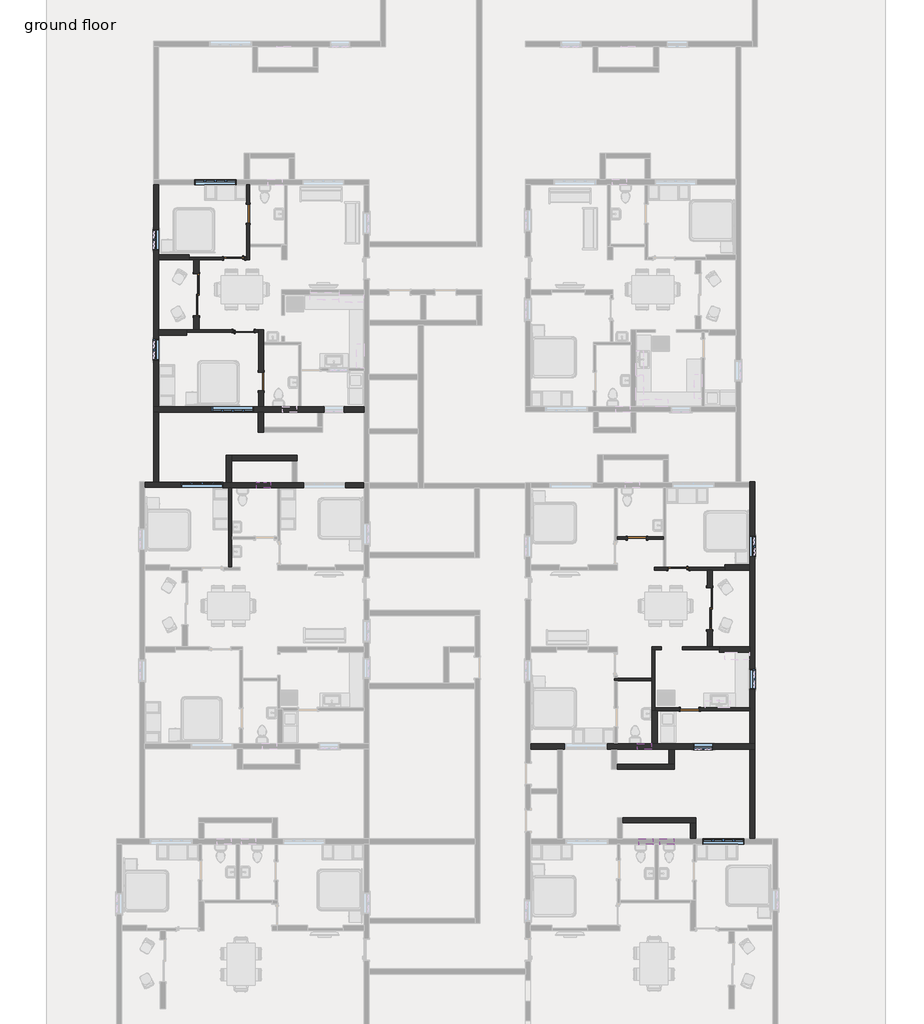
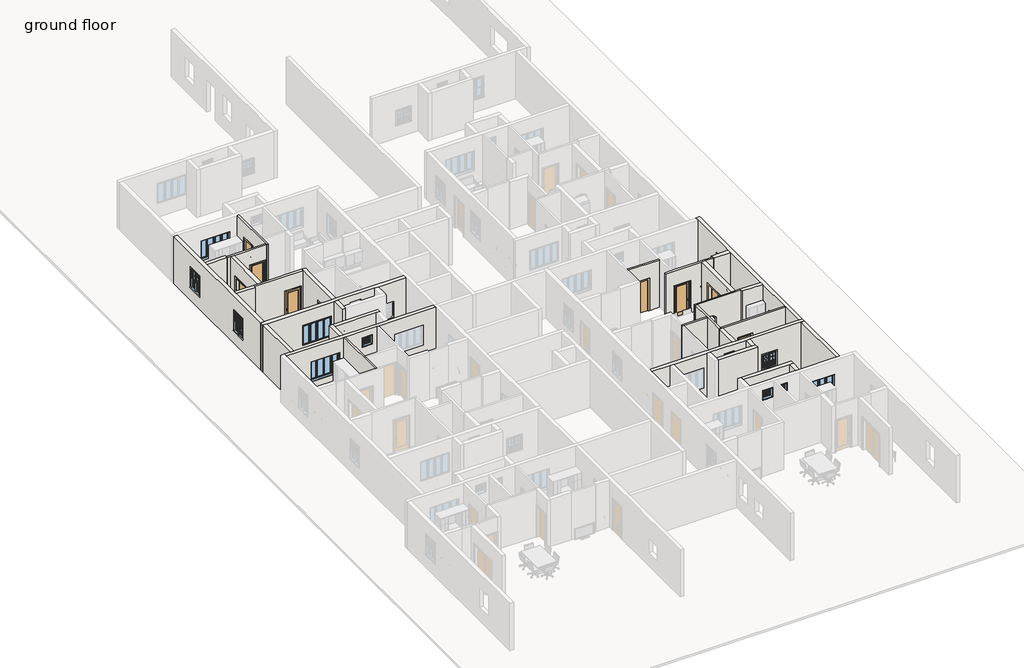
# One storey, part 4 of 16: 32 walls, 13 windows, 9 doors.
"""IFC4 building model written with IfcOpenShell, lengths in millimetres."""

from ifc_helpers import new_model, si_unit, point, frame, origin, place, context, project, spatial, polyline, ellipse_curve, trimmed, outline, extrude, faceted_brep, transform, mapped, element, save
from ifc_brep_helpers import plane_surface, extruded_surface, advanced_brep
from components import door_d4d75d1e, door_a3feeac7, door_38851409, door_d141acb4, door_7b345704, window_ced37e8f, window_5487fb6d, window_f2d8fef0, window_45970670

model = new_model("IFC4")

# Units and contexts
model_context = context("Model", 3, world=origin())
ifc_project = project(units=[si_unit("LENGTHUNIT", "METRE", prefix="MILLI")], contexts=[model_context])

# Site, building, storey
site = spatial("IfcSite", under=ifc_project)
building = spatial("IfcBuilding", under=site)
storey = spatial("IfcBuildingStorey", under=building, Name="ground floor", Elevation=609.6)

# Doors
placement = place(None, origin())
door_shape = door_d4d75d1e(model_context)
element("IfcDoor", 1, ObjectType="Door-Double-Sliding : 72\" x 84\"", at=placement, inside=storey, context=model_context, shape_type="MappedRepresentation", body=[
    mapped(door_shape, transform((67268.6312819, -3471.0113664, 609.6), x_axis=(0.0, -1.0, 0.0), y_axis=(1.0, 0.0, 0.0), z_axis=(0.0, 0.0, 1.0))),
])
element("IfcDoor", 2, ObjectType="Door-Double-Sliding : 72\" x 84\"", at=placement, inside=storey, context=model_context, shape_type="MappedRepresentation", body=[
    mapped(door_shape, transform((44881.526243, 10200.7650652, 609.6), x_axis=(0.0, -1.0, 0.0), y_axis=(1.0, 0.0, 0.0), z_axis=(0.0, 0.0, 1.0))),
])
door_2_shape = door_a3feeac7(model_context)
element("IfcDoor", 3, ObjectType="Door-Interior-Single-1_Panel-Wood : 36\" x 84\"", at=placement, inside=storey, context=model_context, shape_type="MappedRepresentation", body=[
    mapped(door_2_shape, transform((46653.176243, 11785.0900652, 609.6), x_axis=(-1.0, 0.0, 0.0), y_axis=(0.0, -1.0, 0.0), z_axis=(0.0, 0.0, 1.0))),
])
element("IfcDoor", 4, ObjectType="Door-Interior-Single-1_Panel-Wood : 36\" x 84\"", at=placement, inside=storey, context=model_context, shape_type="MappedRepresentation", body=[
    mapped(door_2_shape, transform((47065.926243, 8616.4400652, 609.6), x_axis=(1.0, 0.0, 0.0), y_axis=(0.0, 1.0, 0.0), z_axis=(0.0, 0.0, 1.0))),
])
element("IfcDoor", 5, ObjectType="Door-Interior-Single-1_Panel-Wood : 36\" x 84\"", at=placement, inside=storey, context=model_context, shape_type="MappedRepresentation", body=[
    mapped(door_2_shape, transform((66030.3812819, -1734.2863664, 609.6), x_axis=(-1.0, 0.0, 0.0), y_axis=(0.0, -1.0, 0.0), z_axis=(0.0, 0.0, 1.0))),
])
door_3_shape = door_38851409(model_context)
element("IfcDoor", 6, ObjectType="Single-Flush : 32\" x 84\"", at=placement, inside=storey, context=model_context, shape_type="MappedRepresentation", body=[
    mapped(door_3_shape, transform((64214.2812819, -403.9613664, 609.6), x_axis=(-1.0, 0.0, 0.0), y_axis=(0.0, -1.0, 0.0), z_axis=(0.0, 0.0, 1.0))),
])
door_4_shape = door_d141acb4(model_context)
element("IfcDoor", 7, ObjectType="Single-Flush : 32\" x 84\"", at=placement, inside=storey, context=model_context, shape_type="MappedRepresentation", body=[
    mapped(door_4_shape, transform((47262.776243, 13732.8934407, 609.6), x_axis=(0.0, -1.0, 0.0), y_axis=(1.0, 0.0, 0.0), z_axis=(0.0, 0.0, 1.0))),
])
element("IfcDoor", 8, ObjectType="Single-Flush : 32\" x 84\"", at=placement, inside=storey, context=model_context, shape_type="MappedRepresentation", body=[
    mapped(door_4_shape, transform((66519.3312819, -7858.8613664, 609.6), x_axis=(-1.0, 0.0, 0.0), y_axis=(0.0, -1.0, 0.0), z_axis=(0.0, 0.0, 1.0))),
])
door_5_shape = door_7b345704(model_context)
element("IfcDoor", 9, ObjectType="Single-Flush : 32\" x 84\"", at=placement, inside=storey, context=model_context, shape_type="MappedRepresentation", body=[
    mapped(door_5_shape, transform((47827.926243, 6425.5718163, 609.6), x_axis=(0.0, 1.0, 0.0), y_axis=(-1.0, 0.0, 0.0), z_axis=(0.0, 0.0, 1.0))),
])

# Walls
element("IfcWall", 10, ObjectType="Generic - 4.5\"", at=placement, inside=storey, context=model_context, shape_type="Brep", body=[
    faceted_brep([(47205.626243, 13326.4934407, 2743.2), (47205.626243, 13326.4934407, 609.6), (47205.626243, 11839.0650652, 609.6), (47205.626243, 11724.7650652, 609.6), (47205.626243, 11724.7650652, 3810.0), (47205.626243, 11839.0650652, 3810.0), (47205.626243, 14998.0718163, 3810.0), (47205.626243, 14998.0718163, 609.6), (47205.626243, 14139.2934407, 609.6), (47205.626243, 14139.2934407, 2743.2), (47319.926243, 11724.7650652, 609.6), (47319.926243, 12296.2650652, 609.6), (47319.926243, 12410.5650652, 609.6), (47319.926243, 13326.4934407, 609.6), (47319.926243, 13326.4934407, 2743.2), (47319.926243, 14139.2934407, 2743.2), (47319.926243, 14139.2934407, 609.6), (47319.926243, 14998.0718163, 609.6), (47319.926243, 14998.0718163, 3810.0), (47319.926243, 12410.5650652, 3810.0), (47319.926243, 12296.2650652, 3810.0), (47319.926243, 11724.7650652, 3810.0)], [[[0, 1, 2, 3, 4, 5, 6, 7, 8, 9]], [[10, 11, 12, 13, 14, 15, 16, 17, 18, 19, 20, 21]], [[8, 7, 17, 16]], [[3, 2, 1, 13, 12, 11, 10]], [[6, 5, 4, 21, 20, 19, 18]], [[7, 6, 18, 17]], [[4, 3, 10, 21]], [[14, 13, 1, 0]], [[15, 14, 0, 9]], [[16, 15, 9, 8]]]),
])
element("IfcWall", 11, ObjectType="Generic - 4.5\"", at=placement, inside=storey, context=model_context, shape_type="Brep", body=[
    faceted_brep([(47205.626243, 11724.7650652, 3810.0), (45122.826243, 11724.7650652, 3810.0), (44894.226243, 11724.7650652, 3810.0), (44680.0946956, 11724.7650652, 3810.0), (44680.0946956, 11724.7650652, 609.6), (44894.226243, 11724.7650652, 609.6), (45122.826243, 11724.7650652, 609.6), (46170.576243, 11724.7650652, 609.6), (46170.576243, 11724.7650652, 2768.6), (47135.776243, 11724.7650652, 2768.6), (47135.776243, 11724.7650652, 609.6), (47205.626243, 11724.7650652, 609.6), (44680.0946956, 11839.0650652, 3810.0), (47205.626243, 11839.0650652, 3810.0), (47205.626243, 11839.0650652, 609.6), (47135.776243, 11839.0650652, 609.6), (47135.776243, 11839.0650652, 2768.6), (46170.576243, 11839.0650652, 2768.6), (46170.576243, 11839.0650652, 609.6), (44680.0946956, 11839.0650652, 609.6)], [[[0, 1, 2, 3, 4, 5, 6, 7, 8, 9, 10, 11]], [[12, 13, 14, 15, 16, 17, 18, 19]], [[4, 19, 18, 7, 6, 5]], [[14, 11, 10, 15]], [[3, 2, 1, 0, 13, 12]], [[4, 3, 12, 19]], [[0, 11, 14, 13]], [[17, 8, 7, 18]], [[8, 17, 16, 9]], [[9, 16, 15, 10]]]),
])
element("IfcWall", 12, ObjectType="Generic - 4.5\"", at=placement, inside=storey, context=model_context, shape_type="Brep", body=[
    faceted_brep([(47713.626243, 8562.4650652, 3810.0), (44589.426243, 8562.4650652, 3810.0), (44589.426243, 8562.4650652, 609.6), (46583.326243, 8562.4650652, 609.6), (46583.326243, 8562.4650652, 2768.6), (47548.526243, 8562.4650652, 2768.6), (47548.526243, 8562.4650652, 609.6), (47713.626243, 8562.4650652, 609.6), (44589.426243, 8676.7650652, 3810.0), (44894.226243, 8676.7650652, 3810.0), (45122.826243, 8676.7650652, 3810.0), (47713.626243, 8676.7650652, 3810.0), (47713.626243, 8676.7650652, 609.6), (47548.526243, 8676.7650652, 609.6), (47548.526243, 8676.7650652, 2768.6), (46583.326243, 8676.7650652, 2768.6), (46583.326243, 8676.7650652, 609.6), (45122.826243, 8676.7650652, 609.6), (44894.226243, 8676.7650652, 609.6), (44589.426243, 8676.7650652, 609.6)], [[[0, 1, 2, 3, 4, 5, 6, 7]], [[8, 9, 10, 11, 12, 13, 14, 15, 16, 17, 18, 19]], [[2, 19, 18, 17, 16, 3]], [[12, 7, 6, 13]], [[1, 0, 11, 10, 9, 8]], [[2, 1, 8, 19]], [[0, 7, 12, 11]], [[5, 14, 13, 6]], [[14, 5, 4, 15]], [[15, 4, 3, 16]]]),
])
element("IfcWall", 13, ObjectType="Generic - 4.5\"", at=placement, inside=storey, context=model_context, shape_type="Brep", body=[
    faceted_brep([(46418.226243, 1802.8108651, 609.6), (46418.226243, -1680.3113664, 609.6), (46418.226243, -1680.3113664, 3810.0), (46418.226243, 1802.8108651, 3810.0), (46532.526243, 1802.356101, 609.6), (46532.526243, 1802.356101, 3810.0), (46532.526243, -346.8113664, 3810.0), (46532.526243, -461.1113664, 3810.0), (46532.526243, -1680.3113664, 3810.0), (46532.526243, -1680.3113664, 609.6), (46532.526243, -461.1113664, 609.6), (46532.526243, -346.8113664, 609.6)], [[[0, 1, 2, 3]], [[4, 5, 6, 7, 8, 9, 10, 11]], [[1, 0, 4, 11, 10, 9]], [[3, 2, 8, 7, 6, 5]], [[0, 3, 5, 4]], [[2, 1, 9, 8]]]),
])
element("IfcWall", 14, ObjectType="Generic - 4.5\"", at=placement, inside=storey, context=model_context, shape_type="SweptSolid", body=[
    extrude(outline(polyline([(609.6, 63357.0312819), (609.6, 63807.8812819), (2743.2, 63807.8812819), (2743.2, 64620.6812819), (609.6, 64620.6812819), (609.6, 65363.6312819), (3810.0, 65363.6312819), (3810.0, 63357.0312819), (609.6, 63357.0312819)])), frame((0.0, -461.1113664, 0.0), z_axis=(0.0, 1.0, 0.0), x_axis=(0.0, 0.0, 1.0)), (0.0, 0.0, 1.0), 114.3),
])
element("IfcWall", 15, ObjectType="Generic - 4.5\"", at=placement, inside=storey, context=model_context, shape_type="Brep", body=[
    faceted_brep([(64971.2300724, -1680.3113664, 609.6), (64971.2300724, -1680.3113664, 3810.0), (65363.6312819, -1680.3113664, 3810.0), (65477.9312819, -1680.3113664, 3810.0), (68044.6300724, -1680.3113664, 3810.0), (68044.6300724, -1680.3113664, 609.6), (66512.9812819, -1680.3113664, 609.6), (66512.9812819, -1680.3113664, 2768.6), (65547.7812819, -1680.3113664, 2768.6), (65547.7812819, -1680.3113664, 609.6), (65477.9312819, -1680.3113664, 609.6), (65363.6312819, -1680.3113664, 609.6), (64971.2300724, -1794.6113664, 3810.0), (64971.2300724, -1794.6113664, 609.6), (65547.7812819, -1794.6113664, 609.6), (65547.7812819, -1794.6113664, 2768.6), (66512.9812819, -1794.6113664, 2768.6), (66512.9812819, -1794.6113664, 609.6), (67281.3312819, -1794.6113664, 609.6), (67509.9312819, -1794.6113664, 609.6), (68044.6300724, -1794.6113664, 609.6), (68044.6300724, -1794.6113664, 3810.0), (67509.9312819, -1794.6113664, 3810.0), (67281.3312819, -1794.6113664, 3810.0)], [[[0, 1, 2, 3, 4, 5, 6, 7, 8, 9, 10, 11]], [[12, 13, 14, 15, 16, 17, 18, 19, 20, 21, 22, 23]], [[13, 0, 11, 10, 9, 14]], [[5, 20, 19, 18, 17, 6]], [[1, 0, 13, 12]], [[4, 3, 2, 1, 12, 23, 22, 21]], [[5, 4, 21, 20]], [[8, 15, 14, 9]], [[15, 8, 7, 16]], [[16, 7, 6, 17]]]),
])
element("IfcWall", 16, ObjectType="Generic - 4.5\"", at=placement, inside=storey, context=model_context, shape_type="AdvancedBrep", body=[
    advanced_brep(
    [(65293.7812819, -5147.4113664, 2540.0), (65293.7812819, -5147.4113664, 609.6), (64881.0312819, -5147.4113664, 609.6), (64881.0312819, -5147.4113664, 3810.0), (67281.3312819, -5147.4113664, 3810.0), (67509.9312819, -5147.4113664, 3810.0), (67802.0312819, -5147.4113664, 3810.0), (67802.0312819, -5147.4113664, 609.6), (67509.9312819, -5147.4113664, 609.6), (67281.3312819, -5147.4113664, 609.6), (66208.1812819, -5147.4113664, 609.6), (66208.1812819, -5147.4113664, 2540.0), (64881.0312819, -5261.7113664, 609.6), (64995.3312819, -5261.7113664, 609.6), (65293.7812819, -5261.7113664, 609.6), (65293.7812819, -5261.7113664, 2540.0), (66208.1812819, -5261.7113664, 2540.0), (66208.1812819, -5261.7113664, 609.6), (67802.0312819, -5261.7113664, 609.6), (67802.0312819, -5261.7113664, 3810.0), (64995.3312819, -5261.7113664, 3810.0), (64881.0312819, -5261.7113664, 3810.0)],
    [
        (0, 1),
        (1, 2),
        (2, 3),
        (3, 4),
        (4, 5),
        (5, 6),
        (6, 7),
        (7, 8),
        (8, 9),
        (9, 10),
        (10, 11),
        (11, 0, ellipse_curve(frame((65750.9812819, -5147.4113664, 2540.0), z_axis=(0.0, -1.0, 0.0), x_axis=(-1.0, 0.0, 0.0)), 457.2, 203.2)),
        (12, 13),
        (13, 14),
        (14, 15),
        (15, 16, ellipse_curve(frame((65750.9812819, -5261.7113664, 2540.0), z_axis=(0.0, 1.0, 0.0), x_axis=(-1.0, 0.0, 0.0)), 457.2, 203.2)),
        (16, 17),
        (17, 18),
        (18, 19),
        (19, 20),
        (20, 21),
        (21, 12),
        (1, 14),
        (12, 2),
        (7, 18),
        (17, 10),
        (3, 21),
        (19, 6),
        (15, 0),
        (11, 16),
    ],
    [
        plane_surface(frame((67798.9718682, -5147.4113664, 609.6), z_axis=(0.0, 1.0, 0.0), x_axis=(-1.0, 0.0, 0.0))),
        plane_surface(frame((67798.9718682, -5261.7113664, 609.6), z_axis=(0.0, -1.0, 0.0), x_axis=(1.0, 0.0, 0.0))),
        plane_surface(frame((67802.0312819, -5147.4113664, 609.6), z_axis=(0.0, 0.0, -1.0), x_axis=(0.0, -1.0, 0.0))),
        plane_surface(frame((64938.1812819, -5147.4113664, 3810.0), z_axis=(0.0, 0.0, 1.0), x_axis=(0.0, -1.0, 0.0))),
        plane_surface(frame((67802.0312819, -5147.4113664, 3810.0), z_axis=(1.0, 0.0, 0.0), x_axis=(0.0, -1.0, 0.0))),
        plane_surface(frame((64881.0312819, -5147.4113664, 609.6), z_axis=(-1.0, 0.0, 0.0), x_axis=(0.0, -1.0, 0.0))),
        extruded_surface(trimmed(ellipse_curve(frame((65750.9812819, -5033.1113664, 2540.0), z_axis=(0.0, 1.0, 0.0), x_axis=(-1.0, 0.0, 0.0)), 457.2, 203.2), [point((65293.7812819, -5033.1113664, 2540.0))], [point((66208.1812819, -5033.1113664, 2540.0))], True, "CARTESIAN"), (0.0, -114.29999999999927, 0.0), 114.29999999999927),
        plane_surface(frame((66208.1812819, -5261.7113664, 2540.0), z_axis=(-1.0, 0.0, 0.0), x_axis=(0.0, 1.0, 0.0))),
        plane_surface(frame((65293.7812819, -5261.7113664, 609.6), z_axis=(1.0, 0.0, 0.0), x_axis=(0.0, 1.0, 0.0))),
    ],
    [
        (0, [[1, 2, 3, 4, 5, 6, 7, 8, 9, 10, 11, 12]]),
        (1, [[13, 14, 15, 16, 17, 18, 19, 20, 21, 22]]),
        (2, [[-2, 23, -14, -13, 24]]),
        (2, [[-10, -9, -8, 25, -18, 26]]),
        (3, [[-6, -5, -4, 27, -21, -20, 28]]),
        (4, [[-7, -28, -19, -25]]),
        (5, [[-3, -24, -22, -27]]),
        (6, [[-16, 29, -12, 30]]),
        (7, [[-17, -30, -11, -26]]),
        (8, [[-15, -23, -1, -29]]),
    ],
),
])
element("IfcWall", 17, ObjectType="Generic - 4.5\"", at=placement, inside=storey, context=model_context, shape_type="Brep", body=[
    faceted_brep([(64881.0312819, -5261.7113664, 609.6), (64881.0312819, -6506.3113664, 609.6), (64881.0312819, -6620.6113664, 609.6), (64881.0312819, -7916.0113664, 609.6), (64881.0312819, -7916.0113664, 3810.0), (64881.0312819, -6620.6113664, 3810.0), (64881.0312819, -6506.3113664, 3810.0), (64881.0312819, -5261.7113664, 3810.0), (64995.3312819, -5261.7113664, 609.6), (64995.3312819, -5261.7113664, 3810.0), (64995.3312819, -7801.7113664, 3810.0), (64995.3312819, -7916.0113664, 3810.0), (64995.3312819, -7916.0113664, 609.6), (64995.3312819, -7801.7113664, 609.6)], [[[0, 1, 2, 3, 4, 5, 6, 7]], [[8, 9, 10, 11, 12, 13]], [[3, 2, 1, 0, 8, 13, 12]], [[7, 6, 5, 4, 11, 10, 9]], [[0, 7, 9, 8]], [[4, 3, 12, 11]]]),
])
element("IfcWall", 18, ObjectType="Generic - 4.5\"", at=placement, inside=storey, context=model_context, shape_type="Brep", body=[
    faceted_brep([(64995.3312819, -7916.0113664, 609.6), (65109.6312819, -7916.0113664, 609.6), (66112.9312819, -7916.0113664, 609.6), (66112.9312819, -7916.0113664, 2743.2), (66925.7312819, -7916.0113664, 2743.2), (66925.7312819, -7916.0113664, 609.6), (69135.5312819, -7916.0113664, 609.6), (69135.5312819, -7916.0113664, 3810.0), (65109.6312819, -7916.0113664, 3810.0), (64995.3312819, -7916.0113664, 3810.0), (66112.9312819, -7801.7113664, 2743.2), (66112.9312819, -7801.7113664, 609.6), (64995.3312819, -7801.7113664, 609.6), (64995.3312819, -7801.7113664, 3810.0), (69135.5312819, -7801.7113664, 3810.0), (69135.5312819, -7801.7113664, 609.6), (66925.7312819, -7801.7113664, 609.6), (66925.7312819, -7801.7113664, 2743.2)], [[[0, 1, 2, 3, 4, 5, 6, 7, 8, 9]], [[10, 11, 12, 13, 14, 15, 16, 17]], [[16, 15, 6, 5]], [[12, 11, 2, 1, 0]], [[9, 8, 7, 14, 13]], [[0, 9, 13, 12]], [[7, 6, 15, 14]], [[3, 2, 11, 10]], [[4, 3, 10, 17]], [[5, 4, 17, 16]]]),
])
element("IfcWall", 19, ObjectType="Generic - 4.5\"", at=placement, inside=storey, context=model_context, shape_type="Brep", body=[
    faceted_brep([(64881.0312819, -6506.3113664, 609.6), (63357.0312819, -6506.3113664, 609.6), (63242.7312819, -6506.3113664, 609.6), (63242.7312819, -6506.3113664, 3810.0), (63357.0312819, -6506.3113664, 3810.0), (64881.0312819, -6506.3113664, 3810.0), (64881.0312819, -6620.6113664, 609.6), (64881.0312819, -6620.6113664, 3810.0), (63357.0312819, -6620.6113664, 3810.0), (63242.7312819, -6620.6113664, 3810.0), (63242.7312819, -6620.6113664, 609.6), (63357.0312819, -6620.6113664, 609.6)], [[[0, 1, 2, 3, 4, 5]], [[6, 7, 8, 9, 10, 11]], [[2, 1, 0, 6, 11, 10]], [[5, 4, 3, 9, 8, 7]], [[0, 5, 7, 6]], [[3, 2, 10, 9]]]),
])
element("IfcWall", 20, ObjectType="Generic - 9\"", at=placement, inside=storey, context=model_context, shape_type="Brep", body=[
    faceted_brep([(52311.026243, 5320.6718163, 609.6), (49580.526243, 5320.6718163, 609.6), (49466.226243, 5320.6718163, 609.6), (47942.226243, 5320.6718163, 609.6), (47713.626243, 5320.6718163, 609.6), (43370.226243, 5320.6718163, 609.6), (43141.626243, 5320.6718163, 609.6), (43141.626243, 5320.6718163, 3810.0), (43370.226243, 5320.6718163, 3810.0), (47713.626243, 5320.6718163, 3810.0), (47942.226243, 5320.6718163, 3810.0), (49466.226243, 5320.6718163, 3810.0), (49580.526243, 5320.6718163, 3810.0), (52311.026243, 5320.6718163, 3810.0), (45681.626243, 5320.6718163, 2870.2), (45681.626243, 5320.6718163, 1524.0), (47510.426243, 5320.6718163, 1524.0), (47510.426243, 5320.6718163, 2870.2), (50583.295833, 5320.6718163, 2438.4), (50583.295833, 5320.6718163, 1524.0), (51446.895833, 5320.6718163, 1524.0), (51446.895833, 5320.6718163, 2438.4), (49370.976243, 5320.6718163, 3352.8), (48761.376243, 5320.6718163, 3352.8), (48761.376243, 5320.6718163, 2743.2), (49370.976243, 5320.6718163, 2743.2), (52311.026243, 5092.0718163, 609.6), (52311.026243, 5092.0718163, 3810.0), (50519.795833, 5092.0718163, 3810.0), (50291.195833, 5092.0718163, 3810.0), (47929.526243, 5092.0718163, 3810.0), (47700.926243, 5092.0718163, 3810.0), (43370.226243, 5092.0718163, 3810.0), (43141.626243, 5092.0718163, 3810.0), (43141.626243, 5092.0718163, 609.6), (43370.226243, 5092.0718163, 609.6), (47700.926243, 5092.0718163, 609.6), (47929.526243, 5092.0718163, 609.6), (50291.195833, 5092.0718163, 609.6), (50519.795833, 5092.0718163, 609.6), (45681.626243, 5092.0718163, 2870.2), (47510.426243, 5092.0718163, 2870.2), (47510.426243, 5092.0718163, 1524.0), (45681.626243, 5092.0718163, 1524.0), (50583.295833, 5092.0718163, 2438.4), (51446.895833, 5092.0718163, 2438.4), (51446.895833, 5092.0718163, 1524.0), (50583.295833, 5092.0718163, 1524.0), (49370.976243, 5092.0718163, 3352.8), (49370.976243, 5092.0718163, 2743.2), (48761.376243, 5092.0718163, 2743.2), (48761.376243, 5092.0718163, 3352.8)], [[[0, 1, 2, 3, 4, 5, 6, 7, 8, 9, 10, 11, 12, 13], [14, 15, 16, 17], [18, 19, 20, 21], [22, 23, 24, 25]], [[26, 27, 28, 29, 30, 31, 32, 33, 34, 35, 36, 37, 38, 39], [40, 41, 42, 43], [44, 45, 46, 47], [48, 49, 50, 51]], [[6, 5, 4, 3, 2, 1, 0, 26, 39, 38, 37, 36, 35, 34]], [[13, 12, 11, 10, 9, 8, 7, 33, 32, 31, 30, 29, 28, 27]], [[0, 13, 27, 26]], [[7, 6, 34, 33]], [[15, 14, 40, 43]], [[16, 15, 43, 42]], [[17, 16, 42, 41]], [[14, 17, 41, 40]], [[19, 18, 44, 47]], [[20, 19, 47, 46]], [[21, 20, 46, 45]], [[18, 21, 45, 44]], [[49, 48, 22, 25]], [[50, 49, 25, 24]], [[51, 50, 24, 23]], [[48, 51, 23, 22]]]),
])
element("IfcWall", 21, ObjectType="Generic - 9\"", at=placement, inside=storey, context=model_context, shape_type="Brep", body=[
    faceted_brep([(43370.226243, 5320.6718163, 609.6), (43370.226243, 8448.1650652, 609.6), (43370.226243, 8676.7650652, 609.6), (43370.226243, 11724.7650652, 609.6), (43370.226243, 11953.3650652, 609.6), (43370.226243, 14998.0718163, 609.6), (43370.226243, 14998.0718163, 3810.0), (43370.226243, 11953.3650652, 3810.0), (43370.226243, 11724.7650652, 3810.0), (43370.226243, 8676.7650652, 3810.0), (43370.226243, 8448.1650652, 3810.0), (43370.226243, 5320.6718163, 3810.0), (43370.226243, 7343.2650652, 2844.8), (43370.226243, 8257.6650652, 2844.8), (43370.226243, 8257.6650652, 1524.0), (43370.226243, 7343.2650652, 1524.0), (43370.226243, 12143.8650652, 2844.8), (43370.226243, 13058.2650652, 2844.8), (43370.226243, 13058.2650652, 1524.0), (43370.226243, 12143.8650652, 1524.0), (43141.626243, 5320.6718163, 609.6), (43141.626243, 5320.6718163, 3810.0), (43141.626243, 14998.0718163, 3810.0), (43141.626243, 14998.0718163, 609.6), (43141.626243, 7343.2650652, 2844.8), (43141.626243, 7343.2650652, 1524.0), (43141.626243, 8257.6650652, 1524.0), (43141.626243, 8257.6650652, 2844.8), (43141.626243, 12143.8650652, 2844.8), (43141.626243, 12143.8650652, 1524.0), (43141.626243, 13058.2650652, 1524.0), (43141.626243, 13058.2650652, 2844.8)], [[[0, 1, 2, 3, 4, 5, 6, 7, 8, 9, 10, 11], [12, 13, 14, 15], [16, 17, 18, 19]], [[20, 21, 22, 23], [24, 25, 26, 27], [28, 29, 30, 31]], [[5, 4, 3, 2, 1, 0, 20, 23]], [[11, 10, 9, 8, 7, 6, 22, 21]], [[6, 5, 23, 22]], [[0, 11, 21, 20]], [[25, 24, 12, 15]], [[26, 25, 15, 14]], [[27, 26, 14, 13]], [[24, 27, 13, 12]], [[29, 28, 16, 19]], [[30, 29, 19, 18]], [[31, 30, 18, 17]], [[28, 31, 17, 16]]]),
])
element("IfcWall", 22, ObjectType="Generic - 9\"", at=placement, inside=storey, context=model_context, shape_type="Brep", body=[
    faceted_brep([(43370.226243, 11724.7650652, 609.6), (44680.0946956, 11724.7650652, 609.6), (44680.0946956, 11724.7650652, 3810.0), (43370.226243, 11724.7650652, 3810.0), (43370.226243, 11953.3650652, 609.6), (43370.226243, 11953.3650652, 3810.0), (44680.0946956, 11953.3650652, 3810.0), (44680.0946956, 11953.3650652, 609.6), (44680.0946956, 11839.0650652, 609.6), (44680.0946956, 11839.0650652, 3810.0)], [[[0, 1, 2, 3]], [[4, 5, 6, 7]], [[1, 0, 4, 7, 8]], [[2, 1, 8, 7, 6, 9]], [[3, 2, 9, 6, 5]], [[0, 3, 5, 4]]]),
])
element("IfcWall", 23, ObjectType="Generic - 9\"", at=placement, inside=storey, context=model_context, shape_type="SweptSolid", body=[
    extrude(outline(polyline([(9286.3650652, 2743.2), (9286.3650652, 609.6), (8676.7650652, 609.6), (8676.7650652, 3810.0), (11724.7650652, 3810.0), (11724.7650652, 609.6), (11115.1650652, 609.6), (11115.1650652, 2743.2), (9286.3650652, 2743.2)])), frame((44894.226243, 0.0, 0.0), z_axis=(1.0, 0.0, 0.0), x_axis=(0.0, 1.0, 0.0)), (0.0, 0.0, 1.0), 228.6),
])
element("IfcWall", 24, ObjectType="Generic - 9\"", at=placement, inside=storey, context=model_context, shape_type="Brep", body=[
    faceted_brep([(43370.226243, 8448.1650652, 609.6), (44589.426243, 8448.1650652, 609.6), (44589.426243, 8448.1650652, 3810.0), (43370.226243, 8448.1650652, 3810.0), (43370.226243, 8676.7650652, 609.6), (43370.226243, 8676.7650652, 3810.0), (44589.426243, 8676.7650652, 3810.0), (44589.426243, 8676.7650652, 609.6), (44589.426243, 8562.4650652, 609.6), (44589.426243, 8562.4650652, 3810.0)], [[[0, 1, 2, 3]], [[4, 5, 6, 7]], [[1, 0, 4, 7, 8]], [[2, 1, 8, 7, 6, 9]], [[3, 2, 9, 6, 5]], [[0, 3, 5, 4]]]),
])
element("IfcWall", 25, ObjectType="Generic - 9\"", at=placement, inside=storey, context=model_context, shape_type="Brep", body=[
    faceted_brep([(47713.626243, 8676.7650652, 609.6), (47713.626243, 8562.4650652, 609.6), (47713.626243, 6831.9718163, 609.6), (47713.626243, 6831.9718163, 2743.2), (47713.626243, 6019.1718163, 2743.2), (47713.626243, 6019.1718163, 609.6), (47713.626243, 5320.6718163, 609.6), (47713.626243, 5320.6718163, 3810.0), (47713.626243, 8562.4650652, 3810.0), (47713.626243, 8676.7650652, 3810.0), (47942.226243, 6831.9718163, 2743.2), (47942.226243, 6831.9718163, 609.6), (47942.226243, 8029.0650652, 609.6), (47942.226243, 8143.3650652, 609.6), (47942.226243, 8676.7650652, 609.6), (47942.226243, 8676.7650652, 3810.0), (47942.226243, 8143.3650652, 3810.0), (47942.226243, 8029.0650652, 3810.0), (47942.226243, 5320.6718163, 3810.0), (47942.226243, 5320.6718163, 609.6), (47942.226243, 6019.1718163, 609.6), (47942.226243, 6019.1718163, 2743.2)], [[[0, 1, 2, 3, 4, 5, 6, 7, 8, 9]], [[10, 11, 12, 13, 14, 15, 16, 17, 18, 19, 20, 21]], [[20, 19, 6, 5]], [[14, 13, 12, 11, 2, 1, 0]], [[9, 8, 7, 18, 17, 16, 15]], [[7, 6, 19, 18]], [[0, 9, 15, 14]], [[3, 2, 11, 10]], [[4, 3, 10, 21]], [[5, 4, 21, 20]]]),
])
element("IfcWall", 26, ObjectType="Generic - 9\"", at=placement, inside=storey, context=model_context, shape_type="Brep", body=[
    faceted_brep([(47700.926243, 5092.0718163, 609.6), (47700.926243, 4203.0718163, 609.6), (47700.926243, 4203.0718163, 3810.0), (47700.926243, 5092.0718163, 3810.0), (47929.526243, 5092.0718163, 609.6), (47929.526243, 5092.0718163, 3810.0), (47929.526243, 4431.6718163, 3810.0), (47929.526243, 4203.0718163, 3810.0), (47929.526243, 4203.0718163, 609.6), (47929.526243, 4431.6718163, 609.6)], [[[0, 1, 2, 3]], [[4, 5, 6, 7, 8, 9]], [[1, 0, 4, 9, 8]], [[3, 2, 7, 6, 5]], [[0, 3, 5, 4]], [[2, 1, 8, 7]]]),
])
element("IfcWall", 27, ObjectType="Generic - 9\"", at=placement, inside=storey, context=model_context, shape_type="Brep", body=[
    faceted_brep([(52311.026243, 2007.967056, 609.6), (49401.9107305, 2019.5415219, 609.6), (49173.3107305, 2020.4510502, 609.6), (46532.526243, 2030.9579103, 609.6), (46303.926243, 2031.8674386, 609.6), (43370.226243, 2043.5397185, 609.6), (43141.626243, 2044.4492469, 609.6), (42760.626243, 2045.9651274, 609.6), (42760.626243, 2045.9651274, 3810.0), (43141.626243, 2044.4492469, 3810.0), (43370.226243, 2043.5397185, 3810.0), (46303.926243, 2031.8674386, 3810.0), (46532.526243, 2030.9579103, 3810.0), (49173.3107305, 2020.4510502, 3810.0), (49401.9107305, 2019.5415219, 3810.0), (52311.026243, 2007.967056, 3810.0), (46176.342017, 2032.3750566, 2870.2), (44347.5564917, 2039.6512254, 2870.2), (44347.5564917, 2039.6512254, 1524.0), (46176.342017, 2032.3750566, 1524.0), (51510.2997989, 2011.1528975, 2870.2), (49681.5142737, 2018.4290663, 2870.2), (49681.5142737, 2018.4290663, 1524.0), (51510.2997989, 2011.1528975, 1524.0), (47624.1305578, 2026.6147563, 3352.8), (47624.1305578, 2026.6147563, 2743.2), (48233.7257329, 2024.1893667, 2743.2), (48233.7257329, 2024.1893667, 3352.8), (52311.026243, 1779.3652466, 609.6), (52311.026243, 1779.3652466, 3810.0), (48653.426243, 1793.9176995, 3810.0), (48539.126243, 1794.3724636, 3810.0), (46532.526243, 1802.356101, 3810.0), (46418.226243, 1802.8108651, 3810.0), (42760.626243, 1817.363318, 3810.0), (42760.626243, 1817.363318, 609.6), (46418.226243, 1802.8108651, 609.6), (46532.526243, 1802.356101, 609.6), (48539.126243, 1794.3724636, 609.6), (48653.426243, 1793.9176995, 609.6), (46175.4324959, 1803.7768659, 2870.2), (46175.4324959, 1803.7768659, 1524.0), (44346.6469706, 1811.0530348, 1524.0), (44346.6469706, 1811.0530348, 2870.2), (51509.3902778, 1782.5547068, 2870.2), (51509.3902778, 1782.5547068, 1524.0), (49680.6047526, 1789.8308757, 1524.0), (49680.6047526, 1789.8308757, 2870.2), (47623.2210367, 1798.0165656, 3352.8), (48232.8162118, 1795.591176, 3352.8), (48232.8162118, 1795.591176, 2743.2), (47623.2210367, 1798.0165656, 2743.2)], [[[0, 1, 2, 3, 4, 5, 6, 7, 8, 9, 10, 11, 12, 13, 14, 15], [16, 17, 18, 19], [20, 21, 22, 23], [24, 25, 26, 27]], [[28, 29, 30, 31, 32, 33, 34, 35, 36, 37, 38, 39], [40, 41, 42, 43], [44, 45, 46, 47], [48, 49, 50, 51]], [[7, 6, 5, 4, 3, 2, 1, 0, 28, 39, 38, 37, 36, 35]], [[15, 14, 13, 12, 11, 10, 9, 8, 34, 33, 32, 31, 30, 29]], [[8, 7, 35, 34]], [[0, 15, 29, 28]], [[41, 40, 16, 19]], [[42, 41, 19, 18]], [[43, 42, 18, 17]], [[40, 43, 17, 16]], [[45, 44, 20, 23]], [[46, 45, 23, 22]], [[47, 46, 22, 21]], [[44, 47, 21, 20]], [[25, 24, 48, 51]], [[26, 25, 51, 50]], [[27, 26, 50, 49]], [[24, 27, 49, 48]]]),
])
element("IfcWall", 28, ObjectType="Generic - 9\"", at=placement, inside=storey, context=model_context, shape_type="Brep", body=[
    faceted_brep([(59585.1312819, -9600.7424723, 609.6), (60751.0016338, -9600.7424723, 609.6), (60979.6016338, -9600.7424723, 609.6), (63108.7268416, -9600.7424723, 609.6), (63337.3268416, -9600.7424723, 609.6), (65622.4515239, -9600.7424723, 609.6), (65851.0515239, -9600.7424723, 609.6), (69135.5312819, -9600.7424723, 609.6), (69364.1312819, -9600.7424723, 609.6), (69364.1312819, -9600.7424723, 3810.0), (69135.5312819, -9600.7424723, 3810.0), (65851.0515239, -9600.7424723, 3810.0), (65622.4515239, -9600.7424723, 3810.0), (63337.3268416, -9600.7424723, 3810.0), (63108.7268416, -9600.7424723, 3810.0), (60979.6016338, -9600.7424723, 3810.0), (60751.0016338, -9600.7424723, 3810.0), (59585.1312819, -9600.7424723, 3810.0), (61089.4268416, -9600.7424723, 2870.2), (62918.2268416, -9600.7424723, 2870.2), (62918.2268416, -9600.7424723, 1524.0), (61089.4268416, -9600.7424723, 1524.0), (66676.5515239, -9600.7424723, 2438.4), (67540.1515239, -9600.7424723, 2438.4), (67540.1515239, -9600.7424723, 1524.0), (66676.5515239, -9600.7424723, 1524.0), (64842.9312819, -9600.7424723, 3352.8), (64842.9312819, -9600.7424723, 2743.2), (64233.3312819, -9600.7424723, 2743.2), (64233.3312819, -9600.7424723, 3352.8), (59585.1312819, -9372.1424723, 609.6), (59585.1312819, -9372.1424723, 3810.0), (63242.7312819, -9372.1424723, 3810.0), (63357.0312819, -9372.1424723, 3810.0), (64881.0312819, -9372.1424723, 3810.0), (65109.6312819, -9372.1424723, 3810.0), (69135.5312819, -9372.1424723, 3810.0), (69364.1312819, -9372.1424723, 3810.0), (69364.1312819, -9372.1424723, 609.6), (69135.5312819, -9372.1424723, 609.6), (65109.6312819, -9372.1424723, 609.6), (64881.0312819, -9372.1424723, 609.6), (63357.0312819, -9372.1424723, 609.6), (63242.7312819, -9372.1424723, 609.6), (61089.4268416, -9372.1424723, 2870.2), (61089.4268416, -9372.1424723, 1524.0), (62918.2268416, -9372.1424723, 1524.0), (62918.2268416, -9372.1424723, 2870.2), (66676.5515239, -9372.1424723, 2438.4), (66676.5515239, -9372.1424723, 1524.0), (67540.1515239, -9372.1424723, 1524.0), (67540.1515239, -9372.1424723, 2438.4), (64842.9312819, -9372.1424723, 3352.8), (64233.3312819, -9372.1424723, 3352.8), (64233.3312819, -9372.1424723, 2743.2), (64842.9312819, -9372.1424723, 2743.2)], [[[0, 1, 2, 3, 4, 5, 6, 7, 8, 9, 10, 11, 12, 13, 14, 15, 16, 17], [18, 19, 20, 21], [22, 23, 24, 25], [26, 27, 28, 29]], [[30, 31, 32, 33, 34, 35, 36, 37, 38, 39, 40, 41, 42, 43], [44, 45, 46, 47], [48, 49, 50, 51], [52, 53, 54, 55]], [[8, 7, 6, 5, 4, 3, 2, 1, 0, 30, 43, 42, 41, 40, 39, 38]], [[17, 16, 15, 14, 13, 12, 11, 10, 9, 37, 36, 35, 34, 33, 32, 31]], [[0, 17, 31, 30]], [[9, 8, 38, 37]], [[45, 44, 18, 21]], [[46, 45, 21, 20]], [[47, 46, 20, 19]], [[44, 47, 19, 18]], [[49, 48, 22, 25]], [[50, 49, 25, 24]], [[51, 50, 24, 23]], [[48, 51, 23, 22]], [[27, 26, 52, 55]], [[28, 27, 55, 54]], [[29, 28, 54, 53]], [[26, 29, 53, 52]]]),
])
element("IfcWall", 29, ObjectType="Generic - 9\"", at=placement, inside=storey, context=model_context, shape_type="Brep", body=[
    faceted_brep([(69364.1312819, -9372.1424723, 609.6), (69364.1312819, 2046.8746557, 609.6), (69364.1312819, 2046.8746557, 3810.0), (69364.1312819, -9372.1424723, 3810.0), (69364.1312819, -308.7113664, 2844.8), (69364.1312819, -308.7113664, 1524.0), (69364.1312819, -1223.1113664, 1524.0), (69364.1312819, -1223.1113664, 2844.8), (69364.1312819, -6992.0863664, 2438.4), (69364.1312819, -6128.4863664, 2438.4), (69364.1312819, -6128.4863664, 1524.0), (69364.1312819, -6992.0863664, 1524.0), (69135.5312819, -9372.1424723, 609.6), (69135.5312819, -9372.1424723, 3810.0), (69135.5312819, -7916.0113664, 3810.0), (69135.5312819, -7801.7113664, 3810.0), (69135.5312819, -5376.0113664, 3810.0), (69135.5312819, -5147.4113664, 3810.0), (69135.5312819, -1794.6113664, 3810.0), (69135.5312819, -1566.0113664, 3810.0), (69135.5312819, 1817.363318, 3810.0), (69135.5312819, 2045.9651274, 3810.0), (69135.5312819, 2045.9651274, 609.6), (69135.5312819, 1817.363318, 609.6), (69135.5312819, -1566.0113664, 609.6), (69135.5312819, -1794.6113664, 609.6), (69135.5312819, -5147.4113664, 609.6), (69135.5312819, -5376.0113664, 609.6), (69135.5312819, -7801.7113664, 609.6), (69135.5312819, -7916.0113664, 609.6), (69135.5312819, -308.7113664, 2844.8), (69135.5312819, -1223.1113664, 2844.8), (69135.5312819, -1223.1113664, 1524.0), (69135.5312819, -308.7113664, 1524.0), (69135.5312819, -6992.0863664, 2438.4), (69135.5312819, -6992.0863664, 1524.0), (69135.5312819, -6128.4863664, 1524.0), (69135.5312819, -6128.4863664, 2438.4)], [[[0, 1, 2, 3], [4, 5, 6, 7], [8, 9, 10, 11]], [[12, 13, 14, 15, 16, 17, 18, 19, 20, 21, 22, 23, 24, 25, 26, 27, 28, 29], [30, 31, 32, 33], [34, 35, 36, 37]], [[1, 0, 12, 29, 28, 27, 26, 25, 24, 23, 22]], [[3, 2, 21, 20, 19, 18, 17, 16, 15, 14, 13]], [[0, 3, 13, 12]], [[2, 1, 22, 21]], [[5, 4, 30, 33]], [[6, 5, 33, 32]], [[7, 6, 32, 31]], [[4, 7, 31, 30]], [[35, 34, 8, 11]], [[36, 35, 11, 10]], [[37, 36, 10, 9]], [[34, 37, 9, 8]]]),
])
element("IfcWall", 30, ObjectType="Generic - 9\"", at=placement, inside=storey, context=model_context, shape_type="Brep", body=[
    faceted_brep([(68044.6300724, -1794.6113664, 609.6), (69135.5312819, -1794.6113664, 609.6), (69135.5312819, -1794.6113664, 3810.0), (68044.6300724, -1794.6113664, 3810.0), (68044.6300724, -1566.0113664, 609.6), (68044.6300724, -1566.0113664, 3810.0), (69135.5312819, -1566.0113664, 3810.0), (69135.5312819, -1566.0113664, 609.6), (68044.6300724, -1680.3113664, 609.6), (68044.6300724, -1680.3113664, 3810.0)], [[[0, 1, 2, 3]], [[4, 5, 6, 7]], [[1, 0, 8, 4, 7]], [[3, 2, 6, 5, 9]], [[0, 3, 9, 5, 4, 8]], [[2, 1, 7, 6]]]),
])
element("IfcWall", 31, ObjectType="Generic - 9\"", at=placement, inside=storey, context=model_context, shape_type="Brep", body=[
    faceted_brep([(67802.0312819, -5376.0113664, 609.6), (69135.5312819, -5376.0113664, 609.6), (69135.5312819, -5376.0113664, 3810.0), (67802.0312819, -5376.0113664, 3810.0), (67802.0312819, -5147.4113664, 609.6), (67802.0312819, -5147.4113664, 3810.0), (69135.5312819, -5147.4113664, 3810.0), (69135.5312819, -5147.4113664, 609.6), (67802.0312819, -5261.7113664, 609.6), (67802.0312819, -5261.7113664, 3810.0)], [[[0, 1, 2, 3]], [[4, 5, 6, 7]], [[1, 0, 8, 4, 7]], [[3, 2, 6, 5, 9]], [[0, 3, 9, 5, 4, 8]], [[2, 1, 7, 6]]]),
])
element("IfcWall", 32, ObjectType="Generic - 9\"", at=placement, inside=storey, context=model_context, shape_type="Brep", body=[
    faceted_brep([(65109.6312819, -9372.1424723, 609.6), (65109.6312819, -7916.0113664, 609.6), (65109.6312819, -7916.0113664, 3810.0), (65109.6312819, -9372.1424723, 3810.0), (64881.0312819, -9372.1424723, 609.6), (64881.0312819, -9372.1424723, 3810.0), (64881.0312819, -7916.0113664, 3810.0), (64881.0312819, -7916.0113664, 609.6), (64995.3312819, -7916.0113664, 609.6), (64995.3312819, -7916.0113664, 3810.0)], [[[0, 1, 2, 3]], [[4, 5, 6, 7]], [[1, 0, 4, 7, 8]], [[3, 2, 9, 6, 5]], [[0, 3, 5, 4]], [[2, 1, 8, 7, 6, 9]]]),
])
element("IfcWall", 33, ObjectType="Generic - 9\"", at=placement, inside=storey, context=model_context, shape_type="Brep", body=[
    faceted_brep([(63337.3268416, -10476.6021216, 609.6), (65851.0515239, -10476.6021216, 609.6), (65851.0515239, -10476.6021216, 3810.0), (63337.3268416, -10476.6021216, 3810.0), (63337.3268416, -10248.0021216, 609.6), (63337.3268416, -10248.0021216, 3810.0), (65622.4515239, -10248.0021216, 3810.0), (65851.0515239, -10248.0021216, 3810.0), (65851.0515239, -10248.0021216, 609.6), (65622.4515239, -10248.0021216, 609.6)], [[[0, 1, 2, 3]], [[4, 5, 6, 7, 8, 9]], [[1, 0, 4, 9, 8]], [[3, 2, 7, 6, 5]], [[0, 3, 5, 4]], [[2, 1, 8, 7]]]),
])
element("IfcWall", 34, ObjectType="Generic - 9\"", at=placement, inside=storey, context=model_context, shape_type="SweptSolid", body=[
    extrude(outline(polyline([(65851.0515239, -9600.7424723), (65851.0515239, -10248.0021216), (65622.4515239, -10248.0021216), (65622.4515239, -9600.7424723), (65851.0515239, -9600.7424723)])), frame((0.0, 0.0, 609.6), z_axis=(0.0, 0.0, 1.0), x_axis=(1.0, 0.0, 0.0)), (0.0, 0.0, 1.0), 3200.4),
])
element("IfcWall", 35, ObjectType="Generic - 9\"", at=placement, inside=storey, context=model_context, shape_type="SweptSolid", body=[
    extrude(outline(polyline([(-4385.4113664, 2743.2), (-4385.4113664, 609.6), (-5147.4113664, 609.6), (-5147.4113664, 3810.0), (-1794.6113664, 3810.0), (-1794.6113664, 609.6), (-2556.6113664, 609.6), (-2556.6113664, 2743.2), (-4385.4113664, 2743.2)])), frame((67281.3312819, 0.0, 0.0), z_axis=(1.0, 0.0, 0.0), x_axis=(0.0, 1.0, 0.0)), (0.0, 0.0, 1.0), 228.6),
])
element("IfcWall", 36, ObjectType="Generic - 9\"", at=placement, inside=storey, context=model_context, shape_type="Brep", body=[
    faceted_brep([(46532.526243, 2030.9579103, 609.6), (46532.526243, 2979.67086, 609.6), (46532.526243, 3208.27086, 609.6), (46532.526243, 3208.27086, 3810.0), (46532.526243, 2979.67086, 3810.0), (46532.526243, 2030.9579103, 3810.0), (46303.926243, 2031.8674386, 609.6), (46303.926243, 2031.8674386, 3810.0), (46303.926243, 3208.27086, 3810.0), (46303.926243, 3208.27086, 609.6)], [[[0, 1, 2, 3, 4, 5]], [[6, 7, 8, 9]], [[2, 1, 0, 6, 9]], [[5, 4, 3, 8, 7]], [[0, 5, 7, 6]], [[3, 2, 9, 8]]]),
])
element("IfcWall", 37, ObjectType="Generic - 9\"", at=placement, inside=storey, context=model_context, shape_type="Brep", body=[
    faceted_brep([(46532.526243, 2979.67086, 609.6), (49173.3107305, 2979.67086, 609.6), (49401.9107305, 2979.67086, 609.6), (49401.9107305, 2979.67086, 3810.0), (49173.3107305, 2979.67086, 3810.0), (46532.526243, 2979.67086, 3810.0), (46532.526243, 3208.27086, 609.6), (46532.526243, 3208.27086, 3810.0), (49401.9107305, 3208.27086, 3810.0), (49401.9107305, 3208.27086, 609.6)], [[[0, 1, 2, 3, 4, 5]], [[6, 7, 8, 9]], [[2, 1, 0, 6, 9]], [[5, 4, 3, 8, 7]], [[0, 5, 7, 6]], [[3, 2, 9, 8]]]),
])
element("IfcWall", 38, ObjectType="Generic - 9\"", at=placement, inside=storey, context=model_context, shape_type="Brep", body=[
    faceted_brep([(63585.6312819, -12818.5206064, 609.6), (66557.4312819, -12818.5206064, 609.6), (66786.0312819, -12818.5206064, 609.6), (66786.0312819, -12818.5206064, 3810.0), (66557.4312819, -12818.5206064, 3810.0), (63585.6312819, -12818.5206064, 3810.0), (63585.6312819, -12589.9206064, 609.6), (63585.6312819, -12589.9206064, 3810.0), (66786.0312819, -12589.9206064, 3810.0), (66786.0312819, -12589.9206064, 609.6)], [[[0, 1, 2, 3, 4, 5]], [[6, 7, 8, 9]], [[2, 1, 0, 6, 9]], [[5, 4, 3, 8, 7]], [[0, 5, 7, 6]], [[3, 2, 9, 8]]]),
])
element("IfcWall", 39, ObjectType="Generic - 9\"", at=placement, inside=storey, context=model_context, shape_type="SweptSolid", body=[
    extrude(outline(polyline([(66557.4312819, -13513.0365909), (66557.4312819, -12818.5206064), (66786.0312819, -12818.5206064), (66786.0312819, -13513.0365909), (66557.4312819, -13513.0365909)])), frame((0.0, 0.0, 609.6), z_axis=(0.0, 0.0, 1.0), x_axis=(1.0, 0.0, 0.0)), (0.0, 0.0, 1.0), 3200.4),
])
element("IfcWall", 40, ObjectType="Generic - 9\"", at=placement, inside=storey, context=model_context, shape_type="SweptSolid", body=[
    extrude(outline(polyline([(43141.626243, 2044.4492469), (43141.626243, 5092.0718163), (43370.226243, 5092.0718163), (43370.226243, 2043.5397185), (43141.626243, 2044.4492469)])), frame((0.0, 0.0, 609.6), z_axis=(0.0, 0.0, 1.0), x_axis=(1.0, 0.0, 0.0)), (0.0, 0.0, 1.0), 3200.4),
])
element("IfcWall", 41, ObjectType="Generic - 9\"", at=placement, inside=storey, context=model_context, shape_type="SweptSolid", body=[
    extrude(outline(polyline([(69135.5312819, -13513.0365909), (69135.5312819, -9600.7424723), (69364.1312819, -9600.7424723), (69364.1312819, -13513.0365909), (69135.5312819, -13513.0365909)])), frame((0.0, 0.0, 609.6), z_axis=(0.0, 0.0, 1.0), x_axis=(1.0, 0.0, 0.0)), (0.0, 0.0, 1.0), 3200.4),
])

# Windows
window_shape = window_ced37e8f(model_context)
element("IfcWindow", 42, ObjectType="Window-Casement-Double-Awning : 34\" x 36\"", at=placement, inside=storey, context=model_context, shape_type="MappedRepresentation", body=[
    mapped(window_shape, transform((69249.8312819, -6560.2863664, 609.6), x_axis=(0.0, -1.0, 0.0), y_axis=(1.0, 0.0, 0.0), z_axis=(0.0, 0.0, 1.0))),
])
element("IfcWindow", 43, ObjectType="Window-Casement-Double-Awning : 34\" x 36\"", at=placement, inside=storey, context=model_context, shape_type="MappedRepresentation", body=[
    mapped(window_shape, transform((67108.3515239, -9486.4424723, 609.6), x_axis=(-1.0, 0.0, 0.0), y_axis=(0.0, -1.0, 0.0), z_axis=(0.0, 0.0, 1.0))),
])
window_2_shape = window_5487fb6d(model_context)
element("IfcWindow", 44, ObjectType="Window-Casement-Multi-Sash-Horizontal : 72\" x 53\"", at=placement, inside=storey, context=model_context, shape_type="MappedRepresentation", body=[
    mapped(window_2_shape, transform((67989.3562819, -13627.3365909, 609.6), x_axis=(1.0, 0.0, 0.0), y_axis=(0.0, 1.0, 0.0), z_axis=(0.0, 0.0, 1.0))),
])
element("IfcWindow", 45, ObjectType="Window-Casement-Multi-Sash-Horizontal : 72\" x 53\"", at=placement, inside=storey, context=model_context, shape_type="MappedRepresentation", body=[
    mapped(window_2_shape, transform((45261.4944938, 1921.7140457, 609.6), x_axis=(0.9999920851109113, -0.0039786575037375075, 0.0), y_axis=(0.0039786575037375075, 0.9999920851109113, 0.0), z_axis=(0.0, 0.0, 1.0))),
])
element("IfcWindow", 46, ObjectType="Window-Casement-Multi-Sash-Horizontal : 72\" x 53\"", at=placement, inside=storey, context=model_context, shape_type="MappedRepresentation", body=[
    mapped(window_2_shape, transform((46596.026243, 5206.3718163, 609.6), x_axis=(-1.0, 0.0, 0.0), y_axis=(0.0, -1.0, 0.0), z_axis=(0.0, 0.0, 1.0))),
])
element("IfcWindow", 47, ObjectType="Window-Casement-Multi-Sash-Horizontal : 72\" x 53\"", at=placement, inside=storey, context=model_context, shape_type="MappedRepresentation", body=[
    mapped(window_2_shape, transform((45834.026243, 15112.3718163, 609.6), x_axis=(1.0, 0.0, 0.0), y_axis=(0.0, 1.0, 0.0), z_axis=(0.0, 0.0, 1.0))),
])
window_3_shape = window_f2d8fef0(model_context)
element("IfcWindow", 48, ObjectType="Window-Louvers : 24\" x 24\"", at=placement, inside=storey, context=model_context, shape_type="MappedRepresentation", body=[
    mapped(window_3_shape, transform((64538.1312819, -9492.7924723, 1828.8), x_axis=(-1.0, 0.0, 0.0), y_axis=(0.0, -1.0, 0.0), z_axis=(0.0, 0.0, 1.0))),
])
element("IfcWindow", 49, ObjectType="Window-Louvers : 24\" x 24\"", at=placement, inside=storey, context=model_context, shape_type="MappedRepresentation", body=[
    mapped(window_3_shape, transform((65528.7312819, -13620.9865909, 1828.8), x_axis=(1.0, 0.0, 0.0), y_axis=(0.0, 1.0, 0.0), z_axis=(0.0, 0.0, 1.0))),
])
element("IfcWindow", 50, ObjectType="Window-Louvers : 24\" x 24\"", at=placement, inside=storey, context=model_context, shape_type="MappedRepresentation", body=[
    mapped(window_3_shape, transform((64614.3312819, -13620.9865909, 1828.8), x_axis=(1.0, 0.0, 0.0), y_axis=(0.0, 1.0, 0.0), z_axis=(0.0, 0.0, 1.0))),
])
element("IfcWindow", 51, ObjectType="Window-Louvers : 24\" x 24\"", at=placement, inside=storey, context=model_context, shape_type="MappedRepresentation", body=[
    mapped(window_3_shape, transform((47928.4986492, 1917.4529159, 1828.8), x_axis=(0.9999920851109113, -0.0039786575037375075, 0.0), y_axis=(0.0039786575037375075, 0.9999920851109113, 0.0), z_axis=(0.0, 0.0, 1.0))),
])
window_4_shape = window_45970670(model_context)
element("IfcWindow", 52, ObjectType="Window-Single-Hung-Double : 36\" x 52\"", at=placement, inside=storey, context=model_context, shape_type="MappedRepresentation", body=[
    mapped(window_4_shape, transform((69249.8312819, -765.9113664, 609.6), x_axis=(0.0, -1.0, 0.0), y_axis=(1.0, 0.0, 0.0), z_axis=(0.0, 0.0, 1.0))),
])
element("IfcWindow", 53, ObjectType="Window-Single-Hung-Double : 36\" x 52\"", at=placement, inside=storey, context=model_context, shape_type="MappedRepresentation", body=[
    mapped(window_4_shape, transform((43255.926243, 7800.4650652, 609.6), x_axis=(0.0, 1.0, 0.0), y_axis=(-1.0, 0.0, 0.0), z_axis=(0.0, 0.0, 1.0))),
])
element("IfcWindow", 54, ObjectType="Window-Single-Hung-Double : 36\" x 52\"", at=placement, inside=storey, context=model_context, shape_type="MappedRepresentation", body=[
    mapped(window_4_shape, transform((43255.926243, 12601.0650652, 609.6), x_axis=(0.0, 1.0, 0.0), y_axis=(-1.0, 0.0, 0.0), z_axis=(0.0, 0.0, 1.0))),
])

save(model, "model.ifc")

# Revit data of these elements
# Type "Door-Double-Sliding : 72\" x 84\""
#   Type Mark = "12"
#   Construction Type Id = "opn-d45"
#   Assembly Code = "C1020"
#   Analytic Construction = "Wood frame, double glass door "
#   Thickness = 0' - 2"
#   Thermal Resistance (R) = 1.8150 (h·ft²·°F)/BTU
#   Heat Transfer Coefficient (U) = 0.5510 BTU/(h·ft²·°F)
#   Height = 7' - 0"
#   Rail Width = 0' - 2"
#   Stiles = 0' - 2"
#   Trim Projection Ext = 0' - 1"
#   Trim Projection Int = 0' - 1"
#   Trim Width = 0' - 3"
#   Width = 6' - 0"
#   Define Thermal Properties by = 1
#   Glazing = Glass
#   Panel Material = Wood - Birch - Solid Stained Light Low Gloss
#   Trim Material = Paint - Sienna
#   Visual Light Transmittance = 0
#   Solar Heat Gain Coefficient = 0
#   Function = (empty or 0)
#   Wall Closure = (empty or 0)
# Type "Door-Interior-Single-1_Panel-Wood : 36\" x 84\""
#   Type Mark = "8"
#   Assembly Code = "C1020300"
#   Analytic Construction = "Wooden"
#   Top Rail = 0' - 4 11/16"
#   Thickness = 0' - 1 3/8"
#   Thermal Resistance (R) = 2.5876 (h·ft²·°F)/BTU
#   Swing Angle [instance default] = 90.00°
#   Stiles = 0' - 4 3/4"
#   Rough Width = 3' - 2"
#   Rough Height = 7' - 1"
#   Height = 7' - 0"
#   Width = 3' - 0"
#   Heat Transfer Coefficient (U) = 0.3865 BTU/(h·ft²·°F)
#   Bottom Rail = 0' - 9 1/8"
#   Trim Material = Cherry
#   Panel Material = Cherry
#   Frame Material = Cherry
#   Door Handle Material = Aluminum
#   Visual Light Transmittance = 0
#   Solar Heat Gain Coefficient = 0
#   Wall Closure = (empty or 0)
#   Function = (empty or 0)
# Type "Single-Flush : 32\" x 84\""
#   Type Mark = "3"
#   Construction Type Id = "MDOOR"
#   Assembly Code = "C1020"
#   Analytic Construction = "Metal"
#   Thickness = 0' - 2"
#   Heat Transfer Coefficient (U) = 0.651978 BTU/(h·ft²·°F)
#   Height = 7' - 0"
#   Trim Projection Ext = 0' - 1"
#   Trim Projection Int = 0' - 1"
#   Trim Width = 0' - 3"
#   Width = 2' - 8"
#   Define Thermal Properties by = 1
#   Define Thermal Properties by = 1
#   Door Material = Door - Panel
#   Frame Material = Door - Frame
#   Visual Light Transmittance = 0
#   Solar Heat Gain Coefficient = 0
#   Function = (empty or 0)
#   Wall Closure = (empty or 0)
# Type "Generic - 4.5\""
#   Assembly Code = "B2010"
#   Layers, outside or top first: 0' - 4 1/2" no material (function 1)
# Type "Generic - 9\""
#   Assembly Code = "B2010"
#   Layers, outside or top first: 0' - 9" no material (function 1)
# Type "Window-Casement-Double-Awning : 34\" x 36\""
#   Type Mark = "28"
#   Fire Rating = "0.5h"
#   Assembly Code = "B2020100"
#   Analytic Construction = "Double glazing - domestic"
#   Window Inset [instance default] = 0' - 0"
#   Wall Thickness [instance default] = 0' - 6"
#   Interior Wall Closure [instance default] = 0' - 2 1/4"
#   Half Width = 1' - 5"
#   Visual Light Transmittance = 0.81
#   Thermal Resistance (R) = 1.8146 (h·ft²·°F)/BTU
#   Solar Heat Gain Coefficient = 0.76
#   Rough Width = 2' - 10 1/2"
#   Rough Height = 3' - 0 1/2"
#   Open Window Height = 2' - 0"
#   Height = 3' - 0"
#   Heat Transfer Coefficient (U) = 0.5511 BTU/(h·ft²·°F)
#   Frame Extension [instance default] = 0' - 0 1/4"
#   Exterior Wall Closure [instance default] = 0' - 1 1/4"
#   Awning Height = 1' - 0"
#   Extension Jamb [instance default] = 0' - 2 1/4"
#   Default Sill Height = 3' - 0"
#   Width = 2' - 10"
#   Top Muntin Visibility = yes
#   Interior Trim Visibility [instance default] = yes
#   Bottom Muntin Visibility = yes
#   Exterior Trim Visibility [instance default] = yes
#   Extension Jamb Visibility [instance default] = yes
#   Interior Trim Material = Wood - Stained
#   Muntin Pattern = Muntin Pattern_2x2 : Muntin Pattern_2x2
#   Interior Trim = Trim-Window-Interior-Flat : Picture Frame
#   Interior Frame Material = Wood - Stained
#   Exterior Trim Material = Clad - White
#   Glass Panel Material = Glass
#   Exterior Trim = Trim-Window-Exterior-Flat : with Sill
#   Exterior Frame Material = Clad - White
#   Wall Closure = (empty or 0)
# Type "Window-Casement-Multi-Sash-Horizontal : 72\" x 53\""
#   Type Mark = "24"
#   Fire Rating = "0.5h"
#   Assembly Code = "B2020100"
#   Analytic Construction = "Double glazing - domestic"
#   Window Inset [instance default] = 0' - 0 5/8"
#   Wall Thickness [instance default] = 0' - 6"
#   Visual Light Transmittance = 0.81
#   Thermal Resistance (R) = 1.8146 (h·ft²·°F)/BTU
#   Solar Heat Gain Coefficient = 0.76
#   Rough Width = 6' - 0 1/2"
#   Rough Height = 4' - 5 1/2"
#   Open Window Width = 1' - 6"
#   Heat Transfer Coefficient (U) = 0.5511 BTU/(h·ft²·°F)
#   Height = 4' - 5"
#   Frame Gap 3 [instance default] = 0' - 1 83/128"
#   Frame Gap 2 [instance default] = 0' - 0 5/8"
#   Frame Gap 1 = 0' - 1 51/128"
#   Default Sill Height = 3' - 0"
#   Width = 6' - 0"
#   Frame Material = Metal - Aluminum
#   Glass Panel Material = Glass
#   Wall Closure = (empty or 0)
# Type "Window-Louvers : 24\" x 24\""
#   Type Mark = "18"
#   Construction Type Id = "GSP4R"
#   Assembly Code = "B20"
#   Analytic Construction = "1/8 in Pilkington single glazing"
#   Visual Light Transmittance = 0.9
#   Thermal Resistance (R) = 1.53941 (h·ft²·°F)/BTU
#   Solar Heat Gain Coefficient = 0.78
#   Max Height = 1' - 11.74264"
#   Height = 2' - 0"
#   Heat Transfer Coefficient (U) = 0.6496 BTU/(h·ft²·°F)
#   Blade Width [instance default] = 1' - 10 1/2"
#   Blade Vertical Thickness = 0' - 0.35355"
#   Blade Thickness = 0' - 0 1/4"
#   Blade Spacing = 0' - 1 1/2"
#   Blade Height = 0' - 1.85355"
#   Blade Depth = 0' - 3"
#   Blade Angle = 45.00°
#   Default Sill Height = 3' - 0"
#   Trim Projection_Exterior = 0' - 0 1/2"
#   Trim Projection_Interior = 0' - 0 1/2"
#   Trim Width_Exterior = 0' - 1 1/2"
#   Trim Width_Interior = 0' - 1 1/2"
#   Width = 2' - 0"
#   Max Blade Count = 12
#   Define Thermal Properties by = 1
#   Blade Count = 12
#   Frame Material = Birch
#   Louver Material = Birch
#   Trim Exterior Material = Birch
#   Trim Interior Material = Birch
#   Wall Closure = (empty or 0)
# Type "Window-Single-Hung-Double : 36\" x 52\""
#   Type Mark = "27"
#   Fire Rating = "0.5h"
#   Construction Type Id = "DG-DR"
#   Assembly Code = "B2020100"
#   Analytic Construction = "Double glazing - domestic"
#   Wall Thickness [instance default] = 0' - 6"
#   Window Inset [instance default] = 0' - 0"
#   Visual Light Transmittance = 0.81
#   Thermal Resistance (R) = 1.8146 (h·ft²·°F)/BTU
#   Solar Heat Gain Coefficient = 0.76
#   Muntin Width = 1' - 0 1/16"
#   Muntin Height = 1' - 10 1/8"
#   Interior Wall Closure [instance default] = 0' - 1 1/2"
#   Rough Width = 3' - 0 1/2"
#   Rough Height = 4' - 4 1/2"
#   Frame Extension [instance default] = 0' - 1 1/4"
#   Exterior Wall Closure [instance default] = 0' - 0 1/2"
#   Extension Jamb [instance default] = 0' - 1 1/2"
#   Heat Transfer Coefficient (U) = 0.5511 BTU/(h·ft²·°F)
#   Height = 4' - 4"
#   Width = 3' - 0"
#   Top Muntin Visibility = yes
#   Indicator Visibility [instance default] = yes
#   Extension Jamb Visibility [instance default] = yes
#   Interior Trim Visibility [instance default] = yes
#   Exterior Trim Visibility [instance default] = yes
#   Define Thermal Properties by = 1
#   Bottom Muntin Visibility = yes
#   Muntin Pattern = Muntin Pattern_2x2 : Muntin Pattern_2x2
#   Interior Trim = Trim-Window-Interior-Flat : Picture Frame
#   Interior Trim Material = Wood - Stained
#   Exterior Trim Material = Clad - White
#   Exterior Trim = Trim-Window-Exterior-Flat : with Sill
#   Glass Panel Material = Glass
#   Exterior Frame Material = Clad - White
#   Interior Frame Material = Wood - Stained
#   Wall Closure = (empty or 0)
# Elements 1, 2 (IfcDoor, "Door-Double-Sliding : 72\" x 84\"")
#   Phase Created = New Construction
#   Materials on its faces: "Paint - Sienna", "Wood - Birch - Solid Stained Light Low Gloss", "Glass"
# Elements 3, 4, 5 (IfcDoor, "Door-Interior-Single-1_Panel-Wood : 36\" x 84\"")
#   Swing Angle = 90.00°
#   Phase Created = New Construction
#   Materials on its faces: "Cherry", "Aluminum"
# Elements 6, 7, 8, 9 (IfcDoor, "Single-Flush : 32\" x 84\"")
#   Phase Created = New Construction
#   Materials on its faces: "Door - Frame", "Door - Panel"
# Elements 10, 11, 12, 13, 14, 15, 16, 17, 18, 19 (IfcWall, "Generic - 4.5\"")
#   Top Offset = 0' - 0"
#   Base Offset = 0' - 0"
#   wall height = 10' - 6"
#   Phase Created = New Construction
#   Base Constraint = ground floor
#   Top Constraint = 1st floor
#   Materials on its faces: "Default Wall"
# Elements 20, 21, 22, 23, 24, 25, 26, 27, 28, 29, 30, 31, 32, 33, 34, 35, 36, 37, 38, 39, 40, 41 (IfcWall, "Generic - 9\"")
#   Top Offset = 0' - 0"
#   Base Offset = 0' - 0"
#   wall height = 10' - 6"
#   Phase Created = New Construction
#   Base Constraint = ground floor
#   Top Constraint = 1st floor
#   Materials on its faces: "Default Wall"
